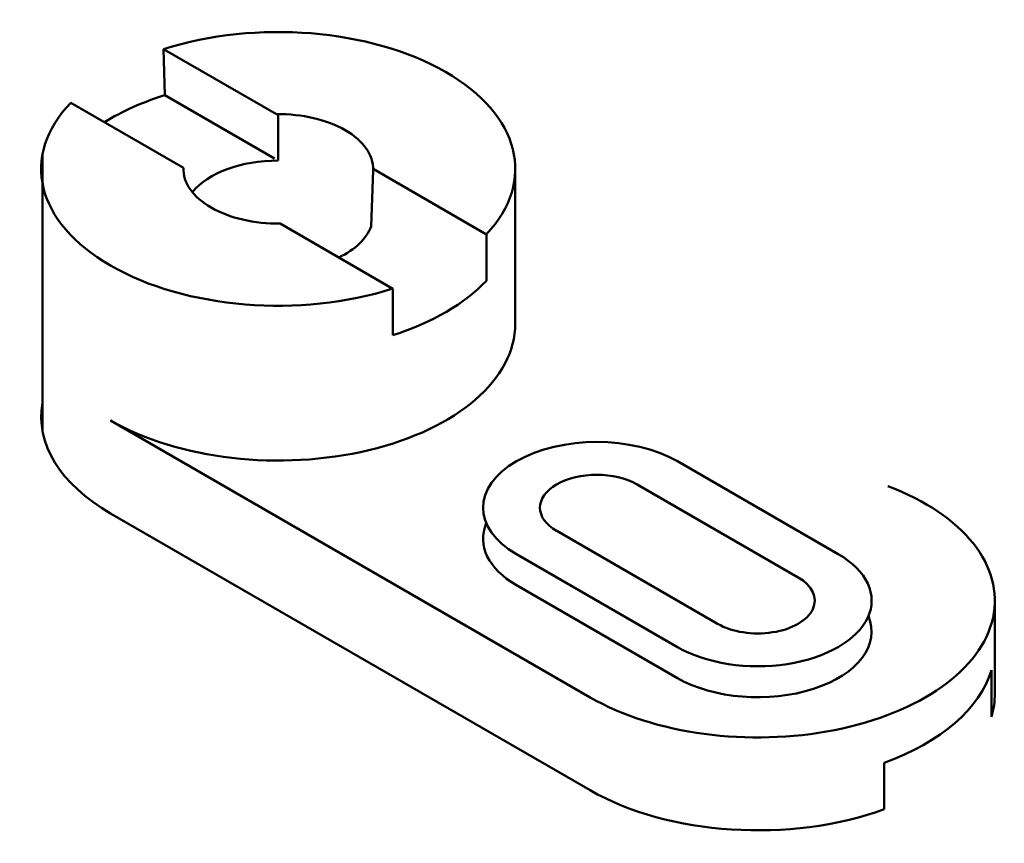
# Model space of a CAD drawing. Units: inches. Extents: x 666 to 20096, y 555 to 16161.
# Tile 1 of 2: x 666 to 793, y 555 to 662. Entities that reach past the tile are written whole.
import ezdxf

# ---------------------------------------------------------------- set-up
doc = ezdxf.new("R2010")
doc.units = ezdxf.units.IN
doc.header["$MEASUREMENT"] = 0
doc.layers.add('M-OUTL', color=7, linetype='Continuous', lineweight=50)

msp = doc.modelspace()

# ---------------------------------------------------------------- linework, layer by layer
at = {"layer": 'M-OUTL'}
for p, q in [((698.82, 649.42), (684.26, 657.82)), ((684.26, 657.82), (684.42, 651.87)), ((698.59, 643.69), (684.42, 651.87)), ((686.82, 642.49), (672.26, 650.89)), ((699.06, 649.42), (699.06, 643.42)), ((668.6, 644.13), (668.6, 608.56)), ((711.31, 642.35), (725.95, 633.89)), ((729.68, 622.35), (729.68, 642.35)), ((711.31, 642.2), (711.06, 634.91)), ((699.31, 635.28), (713.87, 626.87)), ((725.95, 633.89), (725.95, 627.89)), ((713.87, 626.87), (713.87, 620.87)), ((677.41, 609.85), (739.36, 574.08)), ((771.4, 592.58), (750.62, 604.58)), ((766.21, 589.58), (745.42, 601.58)), ((677.41, 597.85), (739.36, 562.08)), ((755.81, 583.58), (735.03, 595.58)), ((750.62, 580.58), (729.83, 592.58)), ((750.62, 576.58), (729.83, 588.58)), ((791.63, 574.58), (791.63, 586.58)), ((791.18, 577.58), (791.18, 571.58)), ((777.32, 565.62), (777.32, 559.62))]:
    msp.add_line(p, q, dxfattribs=at)
for centre, major_axis, start_param, end_param in [((699.06, 642.35), (-30.62, 0), 8.926136, 11.500169), ((699.06, 636.35), (-30.62, 0), 5.211031, 5.534924), ((699.06, 642.35), (-30.62, 0), 5.778591, 8.358576), ((699.06, 642.35), (-12.25, 0), 9.404773, 11.01558), ((699.06, 642.35), (-12.25, 0), 6.26318, 7.873987), ((699.06, 636.35), (-12.25, 0), 4.712389, 5.845036), ((699.06, 636.35), (-12.25, 0), 2.26324, 2.937076), ((699.06, 636.35), (-30.62, 0), 2.075391, 2.642951), ((699.06, 636.35), (-30.62, 0), 2.075391, 2.642951), ((699.06, 622.35), (-30.62, 0), 7.068583, 9.424778), ((699.06, 610.35), (-30.62, 0), 6.181858, 7.068583), ((740.22, 598.58), (-14.7, 0), 3.926991, 7.068583), ((740.22, 598.58), (-7.35, 0), 3.926991, 7.068583), ((761.01, 586.58), (-30.62, 0), 7.068583, 10.41469), ((740.22, 594.58), (-14.7, 0), 6.045244, 7.068583), ((761.01, 586.58), (-14.7, 0), 0.785398, 3.926991), ((761.01, 586.58), (-7.35, 0), 0.785398, 3.926991), ((761.01, 582.58), (-14.7, 0), 0.785398, 3.379534), ((761.01, 580.58), (-30.62, 0), 2.132452, 2.971062), ((761.01, 574.58), (-30.62, 0), 9.254247, 9.424778), ((761.01, 574.58), (-30.62, 0), 7.068583, 8.415637)]:
    msp.add_ellipse(centre, major_axis=major_axis, ratio=0.57735, start_param=start_param, end_param=end_param, dxfattribs=at)

doc.saveas('drawing.dxf')
